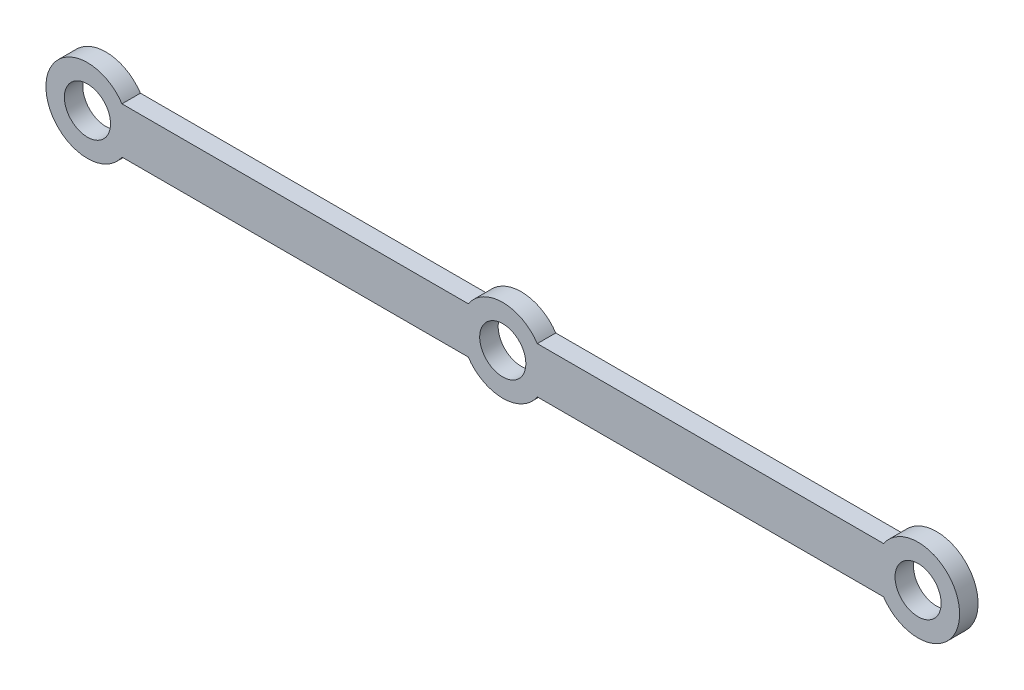
ISO-10303-21;
HEADER;
FILE_DESCRIPTION(('STEP AP214'),'2;1');
FILE_NAME('part.step','',(''),(''),'','','');
FILE_SCHEMA(('AUTOMOTIVE_DESIGN { 1 0 10303 214 1 1 1 1 }'));
ENDSEC;
DATA;
#1=APPLICATION_CONTEXT('core data for automotive mechanical design processes');
#2=APPLICATION_PROTOCOL_DEFINITION('international standard','automotive_design',2000,#1);
#3=PRODUCT_CONTEXT('',#1,'mechanical');
#4=PRODUCT('Part','Part','',(#3));
#5=PRODUCT_RELATED_PRODUCT_CATEGORY('part','',(#4));
#6=PRODUCT_DEFINITION_FORMATION('','',#4);
#7=PRODUCT_DEFINITION_CONTEXT('part definition',#1,'design');
#8=PRODUCT_DEFINITION('design','',#6,#7);
#9=PRODUCT_DEFINITION_SHAPE('','',#8);
#10=(LENGTH_UNIT() NAMED_UNIT(*) SI_UNIT(.MILLI.,.METRE.));
#11=(NAMED_UNIT(*) PLANE_ANGLE_UNIT() SI_UNIT($,.RADIAN.));
#12=(NAMED_UNIT(*) SI_UNIT($,.STERADIAN.) SOLID_ANGLE_UNIT());
#13=UNCERTAINTY_MEASURE_WITH_UNIT(LENGTH_MEASURE(1.E-05),#10,'distance_accuracy_value','');
#14=(GEOMETRIC_REPRESENTATION_CONTEXT(3) GLOBAL_UNCERTAINTY_ASSIGNED_CONTEXT((#13)) GLOBAL_UNIT_ASSIGNED_CONTEXT((#10,
#11,#12)) REPRESENTATION_CONTEXT('',''));
#15=CARTESIAN_POINT('',(0.,0.,0.));
#16=DIRECTION('',(0.,0.,1.));
#17=DIRECTION('',(1.,0.,0.));
#18=AXIS2_PLACEMENT_3D('',#15,#16,#17);
#19=CARTESIAN_POINT('',(0.,0.,1.));
#20=DIRECTION('',(0.,0.,1.));
#21=DIRECTION('',(1.,0.,0.));
#22=AXIS2_PLACEMENT_3D('',#19,#20,#21);
#23=PLANE('',#22);
#24=CARTESIAN_POINT('',(0.,0.,1.));
#25=DIRECTION('',(0.,0.,1.));
#26=DIRECTION('',(1.,0.,0.));
#27=AXIS2_PLACEMENT_3D('',#24,#25,#26);
#28=CIRCLE('',#27,2.5);
#29=CARTESIAN_POINT('',(2.5,0.,1.));
#30=VERTEX_POINT('',#29);
#31=EDGE_CURVE('E189',#30,#30,#28,.T.);
#32=ORIENTED_EDGE('',*,*,#31,.F.);
#33=EDGE_LOOP('',(#32));
#34=FACE_BOUND('',#33,.T.);
#35=CARTESIAN_POINT('',(0.,0.,1.));
#36=DIRECTION('',(0.,0.,1.));
#37=DIRECTION('',(1.,0.,0.));
#38=AXIS2_PLACEMENT_3D('',#35,#36,#37);
#39=CIRCLE('',#38,4.5);
#40=CARTESIAN_POINT('',(3.74165738677394,2.5,1.));
#41=VERTEX_POINT('',#40);
#42=CARTESIAN_POINT('',(-3.74165738677394,2.5,1.));
#43=VERTEX_POINT('',#42);
#44=EDGE_CURVE('E151',#41,#43,#39,.T.);
#45=ORIENTED_EDGE('',*,*,#44,.T.);
#46=DIRECTION('',(-1.,0.,0.));
#47=VECTOR('',#46,1.);
#48=CARTESIAN_POINT('',(-41.2583426132261,2.5,1.));
#49=LINE('',#48,#47);
#50=CARTESIAN_POINT('',(-41.2583426132261,2.5,1.));
#51=VERTEX_POINT('',#50);
#52=EDGE_CURVE('E97',#43,#51,#49,.T.);
#53=ORIENTED_EDGE('',*,*,#52,.T.);
#54=CARTESIAN_POINT('',(-45.,0.,1.));
#55=DIRECTION('',(0.,0.,1.));
#56=DIRECTION('',(1.,0.,0.));
#57=AXIS2_PLACEMENT_3D('',#54,#55,#56);
#58=CIRCLE('',#57,4.5);
#59=CARTESIAN_POINT('',(-41.2583426132261,-2.5,1.));
#60=VERTEX_POINT('',#59);
#61=EDGE_CURVE('E167',#51,#60,#58,.T.);
#62=ORIENTED_EDGE('',*,*,#61,.T.);
#63=DIRECTION('',(1.,0.,0.));
#64=VECTOR('',#63,1.);
#65=CARTESIAN_POINT('',(-41.2583426132261,-2.5,1.));
#66=LINE('',#65,#64);
#67=CARTESIAN_POINT('',(-3.74165738677394,-2.5,1.));
#68=VERTEX_POINT('',#67);
#69=EDGE_CURVE('E177',#60,#68,#66,.T.);
#70=ORIENTED_EDGE('',*,*,#69,.T.);
#71=CARTESIAN_POINT('',(0.,0.,1.));
#72=DIRECTION('',(0.,0.,1.));
#73=DIRECTION('',(1.,0.,0.));
#74=AXIS2_PLACEMENT_3D('',#71,#72,#73);
#75=CIRCLE('',#74,4.5);
#76=CARTESIAN_POINT('',(3.74165738677394,-2.5,1.));
#77=VERTEX_POINT('',#76);
#78=EDGE_CURVE('E119',#68,#77,#75,.T.);
#79=ORIENTED_EDGE('',*,*,#78,.T.);
#80=DIRECTION('',(1.,0.,0.));
#81=VECTOR('',#80,1.);
#82=CARTESIAN_POINT('',(3.74165738677394,-2.5,1.));
#83=LINE('',#82,#81);
#84=CARTESIAN_POINT('',(41.2583426132261,-2.5,1.));
#85=VERTEX_POINT('',#84);
#86=EDGE_CURVE('E115',#77,#85,#83,.T.);
#87=ORIENTED_EDGE('',*,*,#86,.T.);
#88=CARTESIAN_POINT('',(45.,0.,1.));
#89=DIRECTION('',(0.,0.,1.));
#90=DIRECTION('',(1.,0.,0.));
#91=AXIS2_PLACEMENT_3D('',#88,#89,#90);
#92=CIRCLE('',#91,4.5);
#93=CARTESIAN_POINT('',(41.2583426132261,2.5,1.));
#94=VERTEX_POINT('',#93);
#95=EDGE_CURVE('E117',#85,#94,#92,.T.);
#96=ORIENTED_EDGE('',*,*,#95,.T.);
#97=DIRECTION('',(-1.,0.,0.));
#98=VECTOR('',#97,1.);
#99=CARTESIAN_POINT('',(3.74165738677394,2.5,1.));
#100=LINE('',#99,#98);
#101=EDGE_CURVE('E57',#94,#41,#100,.T.);
#102=ORIENTED_EDGE('',*,*,#101,.T.);
#103=EDGE_LOOP('',(#45,#53,#62,#70,#79,#87,#96,#102));
#104=FACE_BOUND('',#103,.T.);
#105=CARTESIAN_POINT('',(-45.,0.,1.));
#106=DIRECTION('',(0.,0.,1.));
#107=DIRECTION('',(1.,0.,0.));
#108=AXIS2_PLACEMENT_3D('',#105,#106,#107);
#109=CIRCLE('',#108,2.5);
#110=CARTESIAN_POINT('',(-42.5,0.,1.));
#111=VERTEX_POINT('',#110);
#112=EDGE_CURVE('E139',#111,#111,#109,.T.);
#113=ORIENTED_EDGE('',*,*,#112,.F.);
#114=EDGE_LOOP('',(#113));
#115=FACE_BOUND('',#114,.T.);
#116=CARTESIAN_POINT('',(45.,0.,1.));
#117=DIRECTION('',(0.,0.,1.));
#118=DIRECTION('',(1.,0.,0.));
#119=AXIS2_PLACEMENT_3D('',#116,#117,#118);
#120=CIRCLE('',#119,2.5);
#121=CARTESIAN_POINT('',(47.5,0.,1.));
#122=VERTEX_POINT('',#121);
#123=EDGE_CURVE('E192',#122,#122,#120,.T.);
#124=ORIENTED_EDGE('',*,*,#123,.F.);
#125=EDGE_LOOP('',(#124));
#126=FACE_BOUND('',#125,.T.);
#127=ADVANCED_FACE('F39',(#34,#104,#115,#126),#23,.T.);
#128=CARTESIAN_POINT('',(0.,0.,-1.));
#129=DIRECTION('',(0.,0.,1.));
#130=DIRECTION('',(1.,0.,0.));
#131=AXIS2_PLACEMENT_3D('',#128,#129,#130);
#132=PLANE('',#131);
#133=CARTESIAN_POINT('',(0.,0.,-1.));
#134=DIRECTION('',(0.,0.,1.));
#135=DIRECTION('',(1.,0.,0.));
#136=AXIS2_PLACEMENT_3D('',#133,#134,#135);
#137=CIRCLE('',#136,4.5);
#138=CARTESIAN_POINT('',(3.74165738677394,2.5,-1.));
#139=VERTEX_POINT('',#138);
#140=CARTESIAN_POINT('',(-3.74165738677394,2.5,-1.));
#141=VERTEX_POINT('',#140);
#142=EDGE_CURVE('E136',#139,#141,#137,.T.);
#143=ORIENTED_EDGE('',*,*,#142,.F.);
#144=DIRECTION('',(-1.,0.,0.));
#145=VECTOR('',#144,1.);
#146=CARTESIAN_POINT('',(3.74165738677394,2.5,-1.));
#147=LINE('',#146,#145);
#148=CARTESIAN_POINT('',(41.2583426132261,2.5,-1.));
#149=VERTEX_POINT('',#148);
#150=EDGE_CURVE('E93',#149,#139,#147,.T.);
#151=ORIENTED_EDGE('',*,*,#150,.F.);
#152=CARTESIAN_POINT('',(45.,0.,-1.));
#153=DIRECTION('',(0.,0.,1.));
#154=DIRECTION('',(1.,0.,0.));
#155=AXIS2_PLACEMENT_3D('',#152,#153,#154);
#156=CIRCLE('',#155,4.5);
#157=CARTESIAN_POINT('',(41.2583426132261,-2.5,-1.));
#158=VERTEX_POINT('',#157);
#159=EDGE_CURVE('E84',#158,#149,#156,.T.);
#160=ORIENTED_EDGE('',*,*,#159,.F.);
#161=DIRECTION('',(1.,0.,0.));
#162=VECTOR('',#161,1.);
#163=CARTESIAN_POINT('',(3.74165738677394,-2.5,-1.));
#164=LINE('',#163,#162);
#165=CARTESIAN_POINT('',(3.74165738677394,-2.5,-1.));
#166=VERTEX_POINT('',#165);
#167=EDGE_CURVE('E127',#166,#158,#164,.T.);
#168=ORIENTED_EDGE('',*,*,#167,.F.);
#169=CARTESIAN_POINT('',(0.,0.,-1.));
#170=DIRECTION('',(0.,0.,1.));
#171=DIRECTION('',(1.,0.,0.));
#172=AXIS2_PLACEMENT_3D('',#169,#170,#171);
#173=CIRCLE('',#172,4.5);
#174=CARTESIAN_POINT('',(-3.74165738677394,-2.5,-1.));
#175=VERTEX_POINT('',#174);
#176=EDGE_CURVE('E148',#175,#166,#173,.T.);
#177=ORIENTED_EDGE('',*,*,#176,.F.);
#178=DIRECTION('',(1.,0.,0.));
#179=VECTOR('',#178,1.);
#180=CARTESIAN_POINT('',(-41.2583426132261,-2.5,-1.));
#181=LINE('',#180,#179);
#182=CARTESIAN_POINT('',(-41.2583426132261,-2.5,-1.));
#183=VERTEX_POINT('',#182);
#184=EDGE_CURVE('E145',#183,#175,#181,.T.);
#185=ORIENTED_EDGE('',*,*,#184,.F.);
#186=CARTESIAN_POINT('',(-45.,0.,-1.));
#187=DIRECTION('',(0.,0.,1.));
#188=DIRECTION('',(1.,0.,0.));
#189=AXIS2_PLACEMENT_3D('',#186,#187,#188);
#190=CIRCLE('',#189,4.5);
#191=CARTESIAN_POINT('',(-41.2583426132261,2.5,-1.));
#192=VERTEX_POINT('',#191);
#193=EDGE_CURVE('E142',#192,#183,#190,.T.);
#194=ORIENTED_EDGE('',*,*,#193,.F.);
#195=DIRECTION('',(-1.,0.,0.));
#196=VECTOR('',#195,1.);
#197=CARTESIAN_POINT('',(-41.2583426132261,2.5,-1.));
#198=LINE('',#197,#196);
#199=EDGE_CURVE('E137',#141,#192,#198,.T.);
#200=ORIENTED_EDGE('',*,*,#199,.F.);
#201=EDGE_LOOP('',(#143,#151,#160,#168,#177,#185,#194,#200));
#202=FACE_BOUND('',#201,.T.);
#203=CARTESIAN_POINT('',(-45.,0.,-1.));
#204=DIRECTION('',(0.,0.,1.));
#205=DIRECTION('',(1.,0.,0.));
#206=AXIS2_PLACEMENT_3D('',#203,#204,#205);
#207=CIRCLE('',#206,2.5);
#208=CARTESIAN_POINT('',(-42.5,0.,-1.));
#209=VERTEX_POINT('',#208);
#210=EDGE_CURVE('E183',#209,#209,#207,.T.);
#211=ORIENTED_EDGE('',*,*,#210,.T.);
#212=EDGE_LOOP('',(#211));
#213=FACE_BOUND('',#212,.T.);
#214=CARTESIAN_POINT('',(0.,0.,-1.));
#215=DIRECTION('',(0.,0.,1.));
#216=DIRECTION('',(1.,0.,0.));
#217=AXIS2_PLACEMENT_3D('',#214,#215,#216);
#218=CIRCLE('',#217,2.5);
#219=CARTESIAN_POINT('',(2.5,0.,-1.));
#220=VERTEX_POINT('',#219);
#221=EDGE_CURVE('E191',#220,#220,#218,.T.);
#222=ORIENTED_EDGE('',*,*,#221,.T.);
#223=EDGE_LOOP('',(#222));
#224=FACE_BOUND('',#223,.T.);
#225=CARTESIAN_POINT('',(45.,0.,-1.));
#226=DIRECTION('',(0.,0.,1.));
#227=DIRECTION('',(1.,0.,0.));
#228=AXIS2_PLACEMENT_3D('',#225,#226,#227);
#229=CIRCLE('',#228,2.5);
#230=CARTESIAN_POINT('',(47.5,0.,-1.));
#231=VERTEX_POINT('',#230);
#232=EDGE_CURVE('E197',#231,#231,#229,.T.);
#233=ORIENTED_EDGE('',*,*,#232,.T.);
#234=EDGE_LOOP('',(#233));
#235=FACE_BOUND('',#234,.T.);
#236=ADVANCED_FACE('F168',(#202,#213,#224,#235),#132,.F.);
#237=CARTESIAN_POINT('',(0.,0.,1.));
#238=DIRECTION('',(0.,0.,-1.));
#239=DIRECTION('',(-1.,0.,0.));
#240=AXIS2_PLACEMENT_3D('',#237,#238,#239);
#241=CYLINDRICAL_SURFACE('',#240,4.5);
#242=ORIENTED_EDGE('',*,*,#142,.T.);
#243=DIRECTION('',(0.,0.,-1.));
#244=VECTOR('',#243,1.);
#245=CARTESIAN_POINT('',(-3.74165738677394,2.5,1.));
#246=LINE('',#245,#244);
#247=EDGE_CURVE('E11',#43,#141,#246,.T.);
#248=ORIENTED_EDGE('',*,*,#247,.F.);
#249=ORIENTED_EDGE('',*,*,#44,.F.);
#250=DIRECTION('',(0.,0.,-1.));
#251=VECTOR('',#250,1.);
#252=CARTESIAN_POINT('',(3.74165738677394,2.5,1.));
#253=LINE('',#252,#251);
#254=EDGE_CURVE('E135',#41,#139,#253,.T.);
#255=ORIENTED_EDGE('',*,*,#254,.T.);
#256=EDGE_LOOP('',(#242,#248,#249,#255));
#257=FACE_BOUND('',#256,.T.);
#258=ADVANCED_FACE('F41',(#257),#241,.T.);
#259=CARTESIAN_POINT('',(-41.2583426132261,2.5,1.));
#260=DIRECTION('',(0.,-1.,0.));
#261=DIRECTION('',(0.,0.,-1.));
#262=AXIS2_PLACEMENT_3D('',#259,#260,#261);
#263=PLANE('',#262);
#264=ORIENTED_EDGE('',*,*,#199,.T.);
#265=DIRECTION('',(0.,0.,-1.));
#266=VECTOR('',#265,1.);
#267=CARTESIAN_POINT('',(-41.2583426132261,2.5,1.));
#268=LINE('',#267,#266);
#269=EDGE_CURVE('E48',#51,#192,#268,.T.);
#270=ORIENTED_EDGE('',*,*,#269,.F.);
#271=ORIENTED_EDGE('',*,*,#52,.F.);
#272=ORIENTED_EDGE('',*,*,#247,.T.);
#273=EDGE_LOOP('',(#264,#270,#271,#272));
#274=FACE_BOUND('',#273,.T.);
#275=ADVANCED_FACE('F228',(#274),#263,.F.);
#276=CARTESIAN_POINT('',(-45.,0.,1.));
#277=DIRECTION('',(0.,0.,-1.));
#278=DIRECTION('',(-1.,0.,0.));
#279=AXIS2_PLACEMENT_3D('',#276,#277,#278);
#280=CYLINDRICAL_SURFACE('',#279,4.5);
#281=ORIENTED_EDGE('',*,*,#193,.T.);
#282=DIRECTION('',(0.,0.,-1.));
#283=VECTOR('',#282,1.);
#284=CARTESIAN_POINT('',(-41.2583426132261,-2.5,1.));
#285=LINE('',#284,#283);
#286=EDGE_CURVE('E158',#60,#183,#285,.T.);
#287=ORIENTED_EDGE('',*,*,#286,.F.);
#288=ORIENTED_EDGE('',*,*,#61,.F.);
#289=ORIENTED_EDGE('',*,*,#269,.T.);
#290=EDGE_LOOP('',(#281,#287,#288,#289));
#291=FACE_BOUND('',#290,.T.);
#292=ADVANCED_FACE('F163',(#291),#280,.T.);
#293=CARTESIAN_POINT('',(-41.2583426132261,-2.5,1.));
#294=DIRECTION('',(0.,1.,0.));
#295=DIRECTION('',(0.,0.,1.));
#296=AXIS2_PLACEMENT_3D('',#293,#294,#295);
#297=PLANE('',#296);
#298=ORIENTED_EDGE('',*,*,#184,.T.);
#299=DIRECTION('',(0.,0.,-1.));
#300=VECTOR('',#299,1.);
#301=CARTESIAN_POINT('',(-3.74165738677394,-2.5,1.));
#302=LINE('',#301,#300);
#303=EDGE_CURVE('E154',#68,#175,#302,.T.);
#304=ORIENTED_EDGE('',*,*,#303,.F.);
#305=ORIENTED_EDGE('',*,*,#69,.F.);
#306=ORIENTED_EDGE('',*,*,#286,.T.);
#307=EDGE_LOOP('',(#298,#304,#305,#306));
#308=FACE_BOUND('',#307,.T.);
#309=ADVANCED_FACE('F173',(#308),#297,.F.);
#310=CARTESIAN_POINT('',(0.,0.,1.));
#311=DIRECTION('',(0.,0.,-1.));
#312=DIRECTION('',(-1.,0.,0.));
#313=AXIS2_PLACEMENT_3D('',#310,#311,#312);
#314=CYLINDRICAL_SURFACE('',#313,4.5);
#315=ORIENTED_EDGE('',*,*,#176,.T.);
#316=DIRECTION('',(0.,0.,-1.));
#317=VECTOR('',#316,1.);
#318=CARTESIAN_POINT('',(3.74165738677394,-2.5,1.));
#319=LINE('',#318,#317);
#320=EDGE_CURVE('E130',#77,#166,#319,.T.);
#321=ORIENTED_EDGE('',*,*,#320,.F.);
#322=ORIENTED_EDGE('',*,*,#78,.F.);
#323=ORIENTED_EDGE('',*,*,#303,.T.);
#324=EDGE_LOOP('',(#315,#321,#322,#323));
#325=FACE_BOUND('',#324,.T.);
#326=ADVANCED_FACE('F178',(#325),#314,.T.);
#327=CARTESIAN_POINT('',(3.74165738677394,-2.5,1.));
#328=DIRECTION('',(0.,1.,0.));
#329=DIRECTION('',(-1.,0.,0.));
#330=AXIS2_PLACEMENT_3D('',#327,#328,#329);
#331=PLANE('',#330);
#332=ORIENTED_EDGE('',*,*,#167,.T.);
#333=DIRECTION('',(0.,0.,-1.));
#334=VECTOR('',#333,1.);
#335=CARTESIAN_POINT('',(41.2583426132261,-2.5,1.));
#336=LINE('',#335,#334);
#337=EDGE_CURVE('E123',#85,#158,#336,.T.);
#338=ORIENTED_EDGE('',*,*,#337,.F.);
#339=ORIENTED_EDGE('',*,*,#86,.F.);
#340=ORIENTED_EDGE('',*,*,#320,.T.);
#341=EDGE_LOOP('',(#332,#338,#339,#340));
#342=FACE_BOUND('',#341,.T.);
#343=ADVANCED_FACE('F122',(#342),#331,.F.);
#344=CARTESIAN_POINT('',(45.,0.,1.));
#345=DIRECTION('',(0.,0.,-1.));
#346=DIRECTION('',(-1.,0.,0.));
#347=AXIS2_PLACEMENT_3D('',#344,#345,#346);
#348=CYLINDRICAL_SURFACE('',#347,4.5);
#349=ORIENTED_EDGE('',*,*,#159,.T.);
#350=DIRECTION('',(0.,0.,-1.));
#351=VECTOR('',#350,1.);
#352=CARTESIAN_POINT('',(41.2583426132261,2.5,1.));
#353=LINE('',#352,#351);
#354=EDGE_CURVE('E126',#94,#149,#353,.T.);
#355=ORIENTED_EDGE('',*,*,#354,.F.);
#356=ORIENTED_EDGE('',*,*,#95,.F.);
#357=ORIENTED_EDGE('',*,*,#337,.T.);
#358=EDGE_LOOP('',(#349,#355,#356,#357));
#359=FACE_BOUND('',#358,.T.);
#360=ADVANCED_FACE('F128',(#359),#348,.T.);
#361=CARTESIAN_POINT('',(3.74165738677394,2.5,1.));
#362=DIRECTION('',(0.,-1.,0.));
#363=DIRECTION('',(1.,0.,0.));
#364=AXIS2_PLACEMENT_3D('',#361,#362,#363);
#365=PLANE('',#364);
#366=ORIENTED_EDGE('',*,*,#150,.T.);
#367=ORIENTED_EDGE('',*,*,#254,.F.);
#368=ORIENTED_EDGE('',*,*,#101,.F.);
#369=ORIENTED_EDGE('',*,*,#354,.T.);
#370=EDGE_LOOP('',(#366,#367,#368,#369));
#371=FACE_BOUND('',#370,.T.);
#372=ADVANCED_FACE('F217',(#371),#365,.F.);
#373=CARTESIAN_POINT('',(-45.,0.,1.));
#374=DIRECTION('',(0.,0.,-1.));
#375=DIRECTION('',(-1.,0.,0.));
#376=AXIS2_PLACEMENT_3D('',#373,#374,#375);
#377=CYLINDRICAL_SURFACE('',#376,2.5);
#378=ORIENTED_EDGE('',*,*,#112,.T.);
#379=EDGE_LOOP('',(#378));
#380=FACE_BOUND('',#379,.T.);
#381=ORIENTED_EDGE('',*,*,#210,.F.);
#382=EDGE_LOOP('',(#381));
#383=FACE_BOUND('',#382,.T.);
#384=ADVANCED_FACE('F214',(#380,#383),#377,.F.);
#385=CARTESIAN_POINT('',(0.,0.,1.));
#386=DIRECTION('',(0.,0.,-1.));
#387=DIRECTION('',(-1.,0.,0.));
#388=AXIS2_PLACEMENT_3D('',#385,#386,#387);
#389=CYLINDRICAL_SURFACE('',#388,2.5);
#390=ORIENTED_EDGE('',*,*,#31,.T.);
#391=EDGE_LOOP('',(#390));
#392=FACE_BOUND('',#391,.T.);
#393=ORIENTED_EDGE('',*,*,#221,.F.);
#394=EDGE_LOOP('',(#393));
#395=FACE_BOUND('',#394,.T.);
#396=ADVANCED_FACE('F291',(#392,#395),#389,.F.);
#397=CARTESIAN_POINT('',(45.,0.,1.));
#398=DIRECTION('',(0.,0.,-1.));
#399=DIRECTION('',(-1.,0.,0.));
#400=AXIS2_PLACEMENT_3D('',#397,#398,#399);
#401=CYLINDRICAL_SURFACE('',#400,2.5);
#402=ORIENTED_EDGE('',*,*,#123,.T.);
#403=EDGE_LOOP('',(#402));
#404=FACE_BOUND('',#403,.T.);
#405=ORIENTED_EDGE('',*,*,#232,.F.);
#406=EDGE_LOOP('',(#405));
#407=FACE_BOUND('',#406,.T.);
#408=ADVANCED_FACE('F201',(#404,#407),#401,.F.);
#409=CLOSED_SHELL('',(#127,#236,#258,#275,#292,#309,#326,#343,#360,#372,#384,#396,#408));
#410=MANIFOLD_SOLID_BREP('B2',#409);
#411=ADVANCED_BREP_SHAPE_REPRESENTATION('',(#18,#410),#14);
#412=SHAPE_DEFINITION_REPRESENTATION(#9,#411);
ENDSEC;
END-ISO-10303-21;
